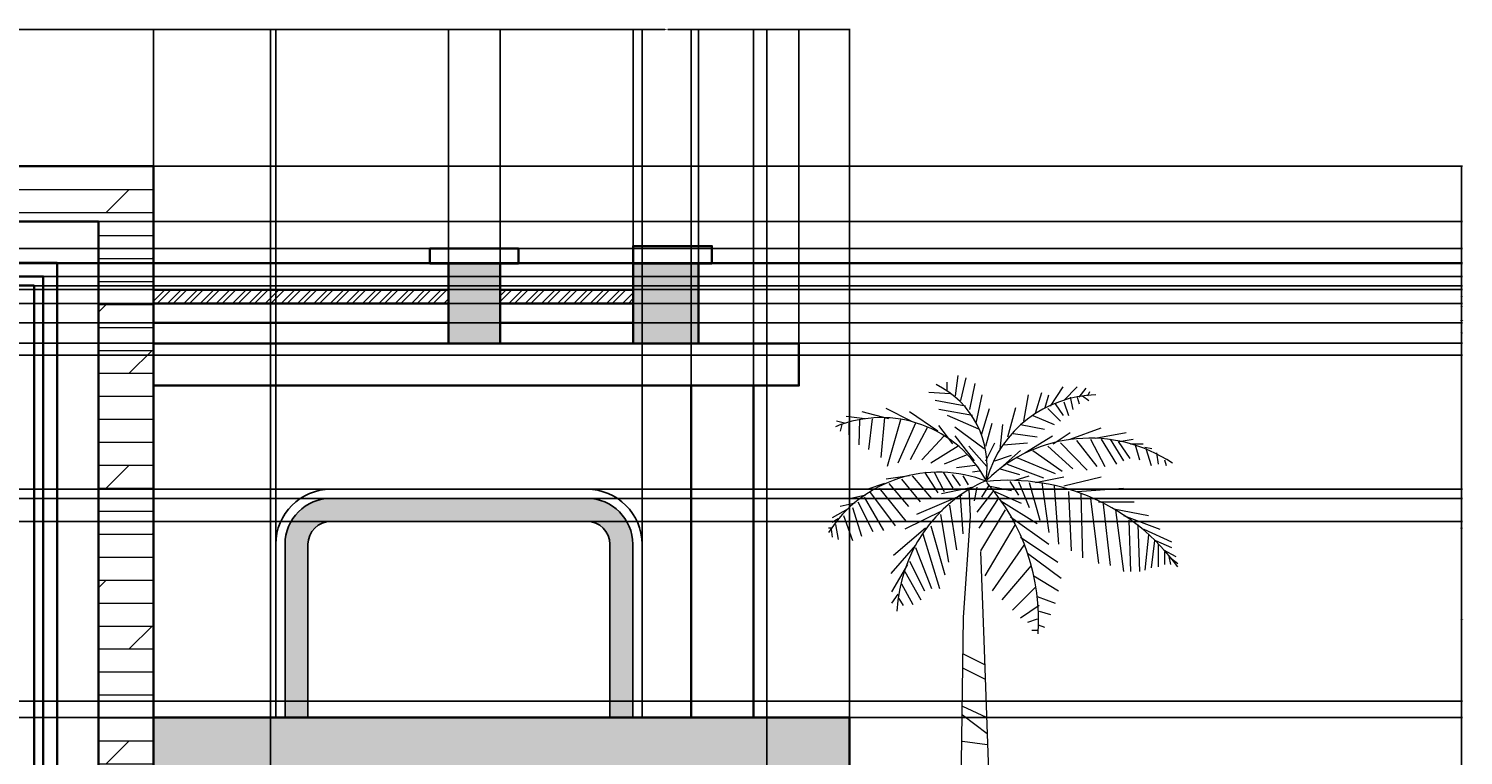
# Model space of a CAD drawing. Units: inches. Extents: x -13 to 630, y -103 to 275.
# Tile 9 of 9: x 318 to 630, y 117 to 275. Entities that reach past the tile are written whole.
import ezdxf

# ---------------------------------------------------------------- set-up
doc = ezdxf.new("R2010")
doc.units = ezdxf.units.IN
doc.header["$MEASUREMENT"] = 0
for name, color, linetype, lineweight in [('A-ANNO-DIMS', 2, 'Continuous', 18), ('A-ELEV', 7, 'Continuous', 35), ('A-ELEV-PATT', 8, 'Continuous', 13), ('A-GLAZ', 4, 'Continuous', 25), ('L-PLNT', 3, 'Continuous', 13)]:
    doc.layers.add(name, color=color, linetype=linetype, lineweight=lineweight)
doc.styles.get("Standard").update_dxf_attribs({"font": 'arial.ttf'})
doc.dimstyles.get("Standard").update_dxf_attribs({"dimtxt": 0.18, "dimasz": 0.18, "dimexe": 0.18, "dimexo": 0.0625, "dimgap": 0.09, "dimtad": 0, "dimtih": 1, "dimtoh": 1, "dimdec": 4, "dimzin": 0, "dimdsep": 46, "dimtxsty": 'Standard', "dimcen": 0.09, "dimadec": 0, "dimazin": 0, "dimtfac": 1, "dimtdec": 4, "dimtofl": 0, "dimtmove": 0, "dimatfit": 3, "dimfxl": 1, "dimtolj": 1, "dimtzin": 0, "dimarcsym": 0})

# ---------------------------------------------------------------- blocks, each defined once
blk = doc.blocks.new('*U2')
for p, q in [((-5.567, 196.707), (-4.987, 201.167)), ((-4.407, 195.716), (-3.247, 200.672)), ((-6.727, 197.202), (-11.366, 197.45)), ((-7.5, 199.68), (-7.5, 197.946)), ((-2.474, 193.733), (-1.315, 199.433)), ((-1.121, 190.759), (0.232, 196.955)), ((9.317, 191.255), (10.283, 196.955)), ((11.829, 192.99), (13.182, 197.45)), ((13.956, 194.229), (14.729, 196.955)), ((15.116, 194.477), (17.822, 198.689)), ((18.015, 195.716), (20.914, 198.689)), ((21.301, 196.459), (22.847, 198.441)), ((22.074, 196.707), (23.427, 195.716)), ((23.234, 196.707), (23.62, 197.698)), ((-15.232, 191.255), (-20.644, 193.981)), ((-3.441, 194.477), (-10.013, 195.716)), ((-1.894, 192.494), (-9.24, 193.733)), ((0.038, 188.281), (1.778, 193.981)), ((5.837, 187.786), (7.577, 194.229)), ((14.536, 193.981), (17.242, 191.255)), ((16.082, 194.972), (17.822, 192.494)), ((18.015, 195.468), (18.981, 192.494)), ((19.368, 196.459), (19.948, 193.733)), ((20.914, 196.459), (21.301, 194.972)), ((-29.729, 190.759), (-31.469, 191.255)), ((-30.309, 190.512), (-30.695, 189.025)), ((-25.283, 191.751), (-29.342, 192.246)), ((-28.763, 190.759), (-28.763, 188.281)), ((-26.443, 191.503), (-26.636, 186.051)), ((-20.064, 191.751), (-25.863, 193.238)), ((-23.737, 191.751), (-24.51, 185.06)), ((-21.031, 191.998), (-21.804, 183.325)), ((-17.551, 191.503), (-20.451, 181.343)), ((-14.265, 190.759), (-18.131, 182.086)), ((-9.433, 189.025), (-15.618, 193.238)), ((-0.541, 189.52), (-7.307, 192.494)), ((1.005, 185.803), (2.358, 190.759)), ((4.098, 185.06), (4.678, 190.512)), ((8.544, 190.512), (13.763, 189.52)), ((11.25, 192.494), (15.889, 190.512)), ((-11.753, 189.768), (-15.425, 182.83)), ((-8.08, 188.034), (-12.912, 182.83)), ((-6.147, 186.299), (-9.24, 190.264)), ((-5.76, 190.016), (0.618, 185.308)), ((-5.76, 188.034), (-1.508, 182.582)), ((6.997, 188.529), (12.216, 187.786)), ((9.51, 184.317), (15.502, 188.034)), ((15.695, 186.299), (19.368, 188.777)), ((19.368, 187.29), (26.133, 189.768)), ((23.814, 187.29), (26.907, 181.343)), ((24.78, 187.538), (31.546, 188.777)), ((26.133, 187.29), (29.419, 181.838)), ((28.066, 187.29), (30.966, 182.582)), ((29.999, 186.795), (33.092, 187.29)), ((-4.987, 185.803), (-10.979, 182.086)), ((-2.668, 185.803), (1.198, 181.343)), ((1.005, 182.582), (2.938, 186.547)), ((4.871, 186.051), (10.09, 186.547)), ((4.871, 181.591), (8.544, 184.812)), ((11.25, 184.812), (17.628, 180.352)), ((14.536, 185.803), (19.948, 180.847)), ((17.242, 186.547), (23.041, 180.599)), ((20.721, 187.042), (25.167, 181.343)), ((29.806, 186.795), (32.319, 183.078)), ((32.512, 186.299), (35.218, 186.299)), ((33.479, 186.051), (34.445, 182.83)), ((35.605, 185.556), (37.151, 185.308)), ((35.798, 185.308), (36.958, 181.591)), ((38.118, 184.317), (38.504, 181.838)), ((-3.247, 183.821), (-8.08, 181.838)), ((-1.315, 181.591), (-5.374, 181.095)), ((2.938, 182.582), (6.61, 183.821)), ((5.644, 181.838), (13.569, 178.865)), ((7.77, 183.325), (16.082, 179.856)), ((39.857, 182.83), (40.244, 181.591)), ((-15.618, 179.36), (-20.644, 178.617)), ((-17.358, 178.617), (-13.299, 173.661)), ((-15.038, 179.36), (-10.786, 174.404)), ((-12.332, 180.104), (-9.433, 175.643)), ((-10.206, 180.104), (-8.08, 175.891)), ((-8.273, 180.104), (-6.147, 176.635)), ((-6.34, 179.608), (-4.6, 177.13)), ((-4.021, 179.36), (-2.861, 177.378)), ((-0.348, 180.352), (-1.894, 180.104)), ((4.098, 180.847), (8.35, 179.608)), ((6.224, 178.121), (8.157, 175.148)), ((7.384, 178.369), (10.476, 179.36)), ((8.157, 178.121), (10.476, 172.422)), ((11.829, 177.874), (18.015, 179.113)), ((18.015, 177.13), (26.133, 179.113)), ((-25.09, 175.148), (-28.376, 174.404)), ((-21.031, 177.626), (-24.897, 176.387)), ((-24.317, 175.891), (-18.711, 168.457)), ((-22.191, 176.635), (-16.391, 169.448)), ((-20.064, 177.626), (-15.812, 172.67)), ((-4.214, 175.148), (-14.072, 170.935)), ((-1.701, 176.882), (-8.66, 175.396)), ((-4.6, 174.9), (-4.021, 166.722)), ((-2.668, 176.387), (-2.376, 170.594)), ((-0.928, 176.882), (-1.508, 173.909)), ((2.551, 175.891), (-0.928, 171.431)), ((1.585, 177.13), (0.038, 174.652)), ((1.585, 177.13), (6.61, 176.139)), ((2.938, 175.891), (8.737, 173.413)), ((10.476, 177.874), (12.796, 169.696)), ((13.182, 177.874), (14.729, 166.97)), ((15.889, 177.13), (16.855, 164.492)), ((18.981, 175.891), (19.561, 163.005)), ((20.914, 175.891), (30.966, 176.635)), ((21.688, 175.396), (22.074, 161.518)), ((-28.956, 172.174), (-32.435, 170.192)), ((-27.409, 173.413), (-30.695, 172.67)), ((-27.989, 172.422), (-26.056, 166.227)), ((-26.829, 173.661), (-23.544, 167.218)), ((-25.476, 174.652), (-21.224, 167.466)), ((-8.466, 171.678), (-16.585, 167.713)), ((-6.92, 172.917), (-5.374, 163.253)), ((3.711, 174.404), (-0.541, 167.961)), ((5.257, 171.926), (-0.155, 163.005)), ((4.291, 173.909), (12.216, 168.953)), ((23.814, 174.404), (25.554, 160.279)), ((25.554, 173.661), (33.285, 173.661)), ((26.52, 173.165), (28.066, 159.784)), ((28.839, 172.174), (36.378, 170.687)), ((29.226, 171.926), (30.966, 158.545)), ((-31.082, 169.944), (-32.435, 169.2)), ((-31.662, 168.705), (-31.082, 165.483)), ((-29.922, 170.687), (-27.989, 165.235)), ((-8.853, 170.935), (-7.113, 160.527)), ((7.384, 168.705), (0.812, 157.553)), ((6.417, 170.439), (14.729, 164.492)), ((30.966, 170.687), (38.891, 167.713)), ((32.126, 169.696), (32.512, 158.545)), ((34.058, 168.705), (34.445, 158.545)), ((-32.628, 167.961), (-33.208, 167.961)), ((-32.628, 167.713), (-32.435, 165.979)), ((-12.139, 167.961), (-19.098, 162.014)), ((-12.719, 166.722), (-9.046, 154.828)), ((-10.979, 168.457), (-7.887, 157.801)), ((8.544, 165.979), (16.662, 160.527)), ((35.412, 167.713), (41.404, 164.988)), ((36.378, 166.474), (35.605, 158.792)), ((-14.265, 164.244), (-19.678, 158.049)), ((-14.265, 163.749), (-10.786, 154.828)), ((9.317, 164.244), (2.358, 154.332)), ((10.09, 162.51), (17.435, 157.058)), ((37.731, 165.235), (36.958, 159.288)), ((37.924, 165.235), (41.404, 163.749)), ((38.504, 164.492), (38.504, 159.536)), ((39.664, 163.253), (42.37, 161.766)), ((39.857, 162.757), (39.857, 160.031)), ((-16.005, 160.031), (-19.484, 154.084)), ((-15.618, 160.775), (-12.332, 154.332)), ((10.863, 159.784), (4.484, 152.35)), ((40.824, 161.766), (41.21, 160.031)), ((41.21, 161.518), (42.757, 160.279)), ((-16.585, 158.545), (-13.106, 152.35)), ((11.443, 157.553), (16.855, 154.332)), ((-18.131, 153.589), (-19.484, 151.606)), ((-17.358, 155.819), (-14.845, 151.358)), ((11.829, 155.075), (6.804, 150.119)), ((12.216, 153.093), (16.082, 151.606)), ((-17.938, 152.597), (-16.972, 151.111)), ((12.603, 151.111), (8.544, 148.385)), ((12.603, 149.872), (15.116, 149.128)), ((12.216, 148.137), (10.09, 147.393)), ((12.409, 146.898), (13.763, 146.402)), ((12.409, 145.659), (11.056, 145.659)), ((-4.081, 140.645), (0.753, 138.261)), ((-4.081, 137.547), (0.753, 135.163)), ((-4.081, 129.205), (1.124, 126.821)), ((-4.081, 127.298), (1.31, 123.246)), ((-4.081, 121.578), (1.31, 120.863))]:
    blk.add_line(p, q)
for points in [[(-2.363, 170.553), (-3.88, 148.505), (-4.988, 69.634), (-3.325, 24.869), (0, 0)], [(-0.116, 162.848), (0.554, 143.532), (2.217, 96.635), (3.88, 44.054), (7.76, 12.079), (11.64, 0)]]:
    blk.add_lwpolyline(points)
for centre, radius, start, end in [((-18.427, 181.448), 19.715, 350.285, 64.11229), ((25.595, 171.567), 25.395, 91.40319, 163.882), ((-21.738, 166.094), 25.899, 27.67115, 112.5305), ((23.687, 155.341), 32.188, 56.19272, 134.3213), ((-9.259, 151.732), 28.386, 68.38311, 147.5322), ((14.394, 148.393), 32.752, 113.7592, 177.4133), ((5.828, 132.718), 45.639, 35.98777, 95.82273), ((-32.8, 147.923), 45.309, 356.1943, 41.37848)]:
    blk.add_arc(centre, radius, start, end)
blk = doc.blocks.new('*D9')
at = {"layer": 'A-ANNO-DIMS', "color": 0, "lineweight": -2, "transparency": 16777216}
for p, q in [((345.31, 5.14), (345.31, 275.01)), ((345.49, 274.83), (357.54, 274.83)), ((370.53, 274.83), (358.47, 274.83)), ((370.71, 5.14), (370.71, 275.01))]:
    blk.add_line(p, q, dxfattribs=at)
at = {"layer": 'A-ANNO-DIMS', "color": 0, "transparency": 16777216}
for points in [[(345.49, 274.86), (345.49, 274.8), (345.31, 274.83)], [(370.53, 274.86), (370.53, 274.8), (370.71, 274.83)]]:
    blk.add_solid(points, dxfattribs=at)
at = {"layer": 'Defpoints', "color": 0, "transparency": 16777216}
for p in [(370.71, 274.83), (345.31, 5.08), (370.71, 5.08)]:
    blk.add_point(p, dxfattribs=at)
at = {"layer": 'A-ANNO-DIMS', "color": 0, "transparency": 16777216, "insert": (358.01, 274.83), "char_height": 0.18, "attachment_point": 5}
blk.add_mtext('\\A1;25.406', dxfattribs=at)
blk = doc.blocks.new('*D10')
at = {"layer": 'A-ANNO-DIMS', "color": 0, "lineweight": -2, "transparency": 16777216}
for p, q in [((478.71, 107.14), (478.71, 275.01)), ((478.89, 274.83), (487.5, 274.83)), ((496.53, 274.83), (487.92, 274.83)), ((496.71, 125.14), (496.71, 275.01))]:
    blk.add_line(p, q, dxfattribs=at)
at = {"layer": 'A-ANNO-DIMS', "color": 0, "transparency": 16777216}
for points in [[(478.89, 274.86), (478.89, 274.8), (478.71, 274.83)], [(496.53, 274.86), (496.53, 274.8), (496.71, 274.83)]]:
    blk.add_solid(points, dxfattribs=at)
at = {"layer": 'Defpoints', "color": 0, "transparency": 16777216}
for p in [(496.71, 274.83), (496.71, 125.08), (478.71, 107.08)]:
    blk.add_point(p, dxfattribs=at)
at = {"layer": 'A-ANNO-DIMS', "color": 0, "transparency": 16777216, "insert": (487.71, 274.83), "char_height": 0.18, "attachment_point": 5}
blk.add_mtext('\\A1;18', dxfattribs=at)
blk = doc.blocks.new('*D13')
at = {"layer": 'A-ANNO-DIMS', "color": 0, "lineweight": -2, "transparency": 16777216}
for p, q in [((345.37, 245.08), (630.03, 245.08)), ((629.85, 244.9), (629.85, 125.26)), ((629.85, 5.26), (629.85, 124.9)), ((496.77, 5.08), (630.03, 5.08))]:
    blk.add_line(p, q, dxfattribs=at)
at = {"layer": 'A-ANNO-DIMS', "color": 0, "transparency": 16777216}
for points in [[(629.82, 244.9), (629.88, 244.9), (629.85, 245.08)], [(629.82, 5.26), (629.88, 5.26), (629.85, 5.08)]]:
    blk.add_solid(points, dxfattribs=at)
at = {"layer": 'Defpoints', "color": 0, "transparency": 16777216}
for p in [(345.31, 245.08), (629.85, 245.08), (496.71, 5.08)]:
    blk.add_point(p, dxfattribs=at)
at = {"layer": 'A-ANNO-DIMS', "color": 0, "transparency": 16777216, "insert": (629.85, 125.08), "char_height": 0.18, "attachment_point": 5}
blk.add_mtext('\\A1;240', dxfattribs=at)
blk = doc.blocks.new('*D14')
at = {"layer": 'A-ANNO-DIMS', "color": 0, "lineweight": -2, "transparency": 16777216}
for p, q in [((345.31, 206.59), (345.31, 275.01)), ((345.49, 274.83), (376.97, 274.83)), ((409.25, 274.83), (377.76, 274.83)), ((409.43, 206.59), (409.43, 275.01))]:
    blk.add_line(p, q, dxfattribs=at)
at = {"layer": 'A-ANNO-DIMS', "color": 0, "transparency": 16777216}
for points in [[(345.49, 274.86), (345.49, 274.8), (345.31, 274.83)], [(409.25, 274.86), (409.25, 274.8), (409.43, 274.83)]]:
    blk.add_solid(points, dxfattribs=at)
at = {"layer": 'Defpoints', "color": 0, "transparency": 16777216}
for p in [(409.43, 274.83), (345.31, 206.53), (409.43, 206.53)]:
    blk.add_point(p, dxfattribs=at)
at = {"layer": 'A-ANNO-DIMS', "color": 0, "transparency": 16777216, "insert": (377.37, 274.83), "char_height": 0.18, "attachment_point": 5}
blk.add_mtext('\\A1;64.12', dxfattribs=at)
blk = doc.blocks.new('*D15')
at = {"layer": 'A-ANNO-DIMS', "color": 0, "lineweight": -2, "transparency": 16777216}
for p, q in [((409.43, 206.59), (409.43, 275.01)), ((409.61, 274.83), (414.6, 274.83)), ((420.5, 274.83), (415.51, 274.83)), ((420.68, 206.59), (420.68, 275.01))]:
    blk.add_line(p, q, dxfattribs=at)
at = {"layer": 'A-ANNO-DIMS', "color": 0, "transparency": 16777216}
for points in [[(409.61, 274.86), (409.61, 274.8), (409.43, 274.83)], [(420.5, 274.86), (420.5, 274.8), (420.68, 274.83)]]:
    blk.add_solid(points, dxfattribs=at)
at = {"layer": 'Defpoints', "color": 0, "transparency": 16777216}
for p in [(420.68, 274.83), (409.43, 206.53), (420.68, 206.53)]:
    blk.add_point(p, dxfattribs=at)
at = {"layer": 'A-ANNO-DIMS', "color": 0, "transparency": 16777216, "insert": (415.06, 274.83), "char_height": 0.18, "attachment_point": 5}
blk.add_mtext('\\A1;11.255', dxfattribs=at)
blk = doc.blocks.new('*D16')
at = {"layer": 'A-ANNO-DIMS', "color": 0, "lineweight": -2, "transparency": 16777216}
for p, q in [((420.68, 206.59), (420.68, 275.01)), ((420.86, 274.83), (434.76, 274.83)), ((449.45, 274.83), (435.55, 274.83)), ((449.63, 206.59), (449.63, 275.01))]:
    blk.add_line(p, q, dxfattribs=at)
at = {"layer": 'A-ANNO-DIMS', "color": 0, "transparency": 16777216}
for points in [[(420.86, 274.86), (420.86, 274.8), (420.68, 274.83)], [(449.45, 274.86), (449.45, 274.8), (449.63, 274.83)]]:
    blk.add_solid(points, dxfattribs=at)
at = {"layer": 'Defpoints', "color": 0, "transparency": 16777216}
for p in [(449.63, 274.83), (420.68, 206.53), (449.63, 206.53)]:
    blk.add_point(p, dxfattribs=at)
at = {"layer": 'A-ANNO-DIMS', "color": 0, "transparency": 16777216, "insert": (435.15, 274.83), "char_height": 0.18, "attachment_point": 5}
blk.add_mtext('\\A1;28.94', dxfattribs=at)
blk = doc.blocks.new('*D17')
at = {"layer": 'A-ANNO-DIMS', "color": 0, "lineweight": -2, "transparency": 16777216}
for p, q in [((449.63, 206.59), (449.63, 275.01)), ((449.81, 274.83), (456.27, 274.83)), ((463.65, 274.83), (457.18, 274.83)), ((463.83, 206.59), (463.83, 275.01))]:
    blk.add_line(p, q, dxfattribs=at)
at = {"layer": 'A-ANNO-DIMS', "color": 0, "transparency": 16777216}
for points in [[(449.81, 274.86), (449.81, 274.8), (449.63, 274.83)], [(463.65, 274.86), (463.65, 274.8), (463.83, 274.83)]]:
    blk.add_solid(points, dxfattribs=at)
at = {"layer": 'Defpoints', "color": 0, "transparency": 16777216}
for p in [(463.83, 274.83), (449.63, 206.53), (463.83, 206.53)]:
    blk.add_point(p, dxfattribs=at)
at = {"layer": 'A-ANNO-DIMS', "color": 0, "transparency": 16777216, "insert": (456.73, 274.83), "char_height": 0.18, "attachment_point": 5}
blk.add_mtext('\\A1;14.203', dxfattribs=at)
blk = doc.blocks.new('*D18')
at = {"layer": 'A-ANNO-DIMS', "color": 0, "lineweight": -2, "transparency": 16777216}
for p, q in [((463.83, 206.59), (463.83, 275.01)), ((464.01, 274.83), (474.28, 274.83)), ((485.49, 274.83), (475.22, 274.83)), ((485.67, 206.59), (485.67, 275.01))]:
    blk.add_line(p, q, dxfattribs=at)
at = {"layer": 'A-ANNO-DIMS', "color": 0, "transparency": 16777216}
for points in [[(464.01, 274.86), (464.01, 274.8), (463.83, 274.83)], [(485.49, 274.86), (485.49, 274.8), (485.67, 274.83)]]:
    blk.add_solid(points, dxfattribs=at)
at = {"layer": 'Defpoints', "color": 0, "transparency": 16777216}
for p in [(485.67, 274.83), (463.83, 206.53), (485.67, 206.53)]:
    blk.add_point(p, dxfattribs=at)
at = {"layer": 'A-ANNO-DIMS', "color": 0, "transparency": 16777216, "insert": (474.75, 274.83), "char_height": 0.18, "attachment_point": 5}
blk.add_mtext('\\A1;21.845', dxfattribs=at)
blk = doc.blocks.new('*D19')
at = {"layer": 'A-ANNO-DIMS', "color": 0, "lineweight": -2, "transparency": 16777216}
for p, q in [((485.67, 206.59), (485.67, 275.01)), ((485.85, 274.83), (490.74, 274.83)), ((496.53, 274.83), (491.65, 274.83)), ((496.71, 125.14), (496.71, 275.01))]:
    blk.add_line(p, q, dxfattribs=at)
at = {"layer": 'A-ANNO-DIMS', "color": 0, "transparency": 16777216}
for points in [[(485.85, 274.86), (485.85, 274.8), (485.67, 274.83)], [(496.53, 274.86), (496.53, 274.8), (496.71, 274.83)]]:
    blk.add_solid(points, dxfattribs=at)
at = {"layer": 'Defpoints', "color": 0, "transparency": 16777216}
for p in [(496.71, 274.83), (485.67, 206.53), (496.71, 125.08)]:
    blk.add_point(p, dxfattribs=at)
at = {"layer": 'A-ANNO-DIMS', "color": 0, "transparency": 16777216, "insert": (491.19, 274.83), "char_height": 0.18, "attachment_point": 5}
blk.add_mtext('\\A1;11.038', dxfattribs=at)
blk = doc.blocks.new('*D20')
at = {"layer": 'A-ANNO-DIMS', "color": 0, "lineweight": -2, "transparency": 16777216}
for p, q in [((345.31, 125.14), (345.31, 275.01)), ((345.49, 274.83), (358.13, 274.83)), ((371.7, 274.83), (359.06, 274.83)), ((371.88, 125.14), (371.88, 275.01))]:
    blk.add_line(p, q, dxfattribs=at)
at = {"layer": 'A-ANNO-DIMS', "color": 0, "transparency": 16777216}
for points in [[(345.49, 274.86), (345.49, 274.8), (345.31, 274.83)], [(371.7, 274.86), (371.7, 274.8), (371.88, 274.83)]]:
    blk.add_solid(points, dxfattribs=at)
at = {"layer": 'Defpoints', "color": 0, "transparency": 16777216}
for p in [(371.88, 274.83), (345.31, 125.08), (371.88, 125.08)]:
    blk.add_point(p, dxfattribs=at)
at = {"layer": 'A-ANNO-DIMS', "color": 0, "transparency": 16777216, "insert": (358.59, 274.83), "char_height": 0.18, "attachment_point": 5}
blk.add_mtext('\\A1;26.576', dxfattribs=at)
blk = doc.blocks.new('*D21')
at = {"layer": 'A-ANNO-DIMS', "color": 0, "lineweight": -2, "transparency": 16777216}
for p, q in [((371.88, 125.14), (371.88, 275.01)), ((372.06, 274.83), (411.32, 274.83)), ((451.37, 274.83), (412.11, 274.83)), ((451.55, 125.14), (451.55, 275.01))]:
    blk.add_line(p, q, dxfattribs=at)
at = {"layer": 'A-ANNO-DIMS', "color": 0, "transparency": 16777216}
for points in [[(372.06, 274.86), (372.06, 274.8), (371.88, 274.83)], [(451.37, 274.86), (451.37, 274.8), (451.55, 274.83)]]:
    blk.add_solid(points, dxfattribs=at)
at = {"layer": 'Defpoints', "color": 0, "transparency": 16777216}
for p in [(451.55, 274.83), (371.88, 125.08), (451.55, 125.08)]:
    blk.add_point(p, dxfattribs=at)
at = {"layer": 'A-ANNO-DIMS', "color": 0, "transparency": 16777216, "insert": (411.72, 274.83), "char_height": 0.18, "attachment_point": 5}
blk.add_mtext('\\A1;79.67', dxfattribs=at)
blk = doc.blocks.new('*D22')
at = {"layer": 'A-ANNO-DIMS', "color": 0, "lineweight": -2, "transparency": 16777216}
for p, q in [((451.55, 125.14), (451.55, 275.01)), ((451.73, 274.83), (456.54, 274.83)), ((462.08, 274.83), (457.27, 274.83)), ((462.26, 125.14), (462.26, 275.01))]:
    blk.add_line(p, q, dxfattribs=at)
at = {"layer": 'A-ANNO-DIMS', "color": 0, "transparency": 16777216}
for points in [[(451.73, 274.86), (451.73, 274.8), (451.55, 274.83)], [(462.08, 274.86), (462.08, 274.8), (462.26, 274.83)]]:
    blk.add_solid(points, dxfattribs=at)
at = {"layer": 'Defpoints', "color": 0, "transparency": 16777216}
for p in [(462.26, 274.83), (451.55, 125.08), (462.26, 125.08)]:
    blk.add_point(p, dxfattribs=at)
at = {"layer": 'A-ANNO-DIMS', "color": 0, "transparency": 16777216, "insert": (456.91, 274.83), "char_height": 0.18, "attachment_point": 5}
blk.add_mtext('\\A1;10.71', dxfattribs=at)
blk = doc.blocks.new('*D23')
at = {"layer": 'A-ANNO-DIMS', "color": 0, "lineweight": -2, "transparency": 16777216}
for p, q in [((462.26, 125.14), (462.26, 275.01)), ((462.44, 274.83), (468.59, 274.83)), ((475.65, 274.83), (469.5, 274.83)), ((475.83, 125.14), (475.83, 275.01))]:
    blk.add_line(p, q, dxfattribs=at)
at = {"layer": 'A-ANNO-DIMS', "color": 0, "transparency": 16777216}
for points in [[(462.44, 274.86), (462.44, 274.8), (462.26, 274.83)], [(475.65, 274.86), (475.65, 274.8), (475.83, 274.83)]]:
    blk.add_solid(points, dxfattribs=at)
at = {"layer": 'Defpoints', "color": 0, "transparency": 16777216}
for p in [(475.83, 274.83), (462.26, 125.08), (475.83, 125.08)]:
    blk.add_point(p, dxfattribs=at)
at = {"layer": 'A-ANNO-DIMS', "color": 0, "transparency": 16777216, "insert": (469.05, 274.83), "char_height": 0.18, "attachment_point": 5}
blk.add_mtext('\\A1;13.574', dxfattribs=at)
blk = doc.blocks.new('*D27')
at = {"layer": 'A-ANNO-DIMS', "color": 0, "lineweight": -2, "transparency": 16777216}
for p, q in [((164.84, 245.14), (164.84, 275.01)), ((165.02, 274.83), (254.62, 274.83)), ((345.13, 274.83), (255.53, 274.83)), ((345.31, 245.14), (345.31, 275.01))]:
    blk.add_line(p, q, dxfattribs=at)
at = {"layer": 'A-ANNO-DIMS', "color": 0, "transparency": 16777216}
for points in [[(165.02, 274.86), (165.02, 274.8), (164.84, 274.83)], [(345.13, 274.86), (345.13, 274.8), (345.31, 274.83)]]:
    blk.add_solid(points, dxfattribs=at)
at = {"layer": 'Defpoints', "color": 0, "transparency": 16777216}
for p in [(345.31, 274.83), (164.84, 245.08), (345.31, 245.08)]:
    blk.add_point(p, dxfattribs=at)
at = {"layer": 'A-ANNO-DIMS', "color": 0, "transparency": 16777216, "insert": (255.08, 274.83), "char_height": 0.18, "attachment_point": 5}
blk.add_mtext('\\A1;180.46', dxfattribs=at)
blk = doc.blocks.new('*D28')
at = {"layer": 'A-ANNO-DIMS', "color": 0, "lineweight": -2, "transparency": 16777216}
for p, q in [((302.59, 128.66), (630.03, 128.66)), ((629.85, 128.48), (629.85, 67.05)), ((629.85, 5.26), (629.85, 66.69)), ((302.59, 5.08), (630.03, 5.08))]:
    blk.add_line(p, q, dxfattribs=at)
at = {"layer": 'A-ANNO-DIMS', "color": 0, "transparency": 16777216}
for points in [[(629.82, 128.48), (629.88, 128.48), (629.85, 128.66)], [(629.82, 5.26), (629.88, 5.26), (629.85, 5.08)]]:
    blk.add_solid(points, dxfattribs=at)
at = {"layer": 'Defpoints', "color": 0, "transparency": 16777216}
for p in [(302.53, 128.66), (629.85, 128.66), (302.53, 5.08)]:
    blk.add_point(p, dxfattribs=at)
at = {"layer": 'A-ANNO-DIMS', "color": 0, "transparency": 16777216, "insert": (629.85, 66.87), "char_height": 0.18, "attachment_point": 5}
blk.add_mtext('\\A1;123.57', dxfattribs=at)
blk = doc.blocks.new('*D29')
at = {"layer": 'A-ANNO-DIMS', "color": 0, "lineweight": -2, "transparency": 16777216}
for p, q in [((302.59, 203.94), (630.03, 203.94)), ((629.85, 203.76), (629.85, 166.48)), ((629.85, 128.84), (629.85, 166.11)), ((302.59, 128.66), (630.03, 128.66))]:
    blk.add_line(p, q, dxfattribs=at)
at = {"layer": 'A-ANNO-DIMS', "color": 0, "transparency": 16777216}
for points in [[(629.82, 203.76), (629.88, 203.76), (629.85, 203.94)], [(629.82, 128.84), (629.88, 128.84), (629.85, 128.66)]]:
    blk.add_solid(points, dxfattribs=at)
at = {"layer": 'Defpoints', "color": 0, "transparency": 16777216}
for p in [(302.53, 203.94), (629.85, 203.94), (302.53, 128.66)]:
    blk.add_point(p, dxfattribs=at)
at = {"layer": 'A-ANNO-DIMS', "color": 0, "transparency": 16777216, "insert": (629.85, 166.3), "char_height": 0.18, "attachment_point": 5}
blk.add_mtext('\\A1;75.28', dxfattribs=at)
blk = doc.blocks.new('*D35')
at = {"layer": 'A-ANNO-DIMS', "color": 0, "lineweight": -2, "transparency": 16777216}
for p, q in [((319.37, 219.08), (630.03, 219.08)), ((629.85, 218.9), (629.85, 211.69)), ((629.85, 204.12), (629.85, 211.33)), ((302.59, 203.94), (630.03, 203.94))]:
    blk.add_line(p, q, dxfattribs=at)
at = {"layer": 'A-ANNO-DIMS', "color": 0, "transparency": 16777216}
for points in [[(629.82, 218.9), (629.88, 218.9), (629.85, 219.08)], [(629.82, 204.12), (629.88, 204.12), (629.85, 203.94)]]:
    blk.add_solid(points, dxfattribs=at)
at = {"layer": 'Defpoints', "color": 0, "transparency": 16777216}
for p in [(319.31, 219.08), (629.85, 219.08), (302.53, 203.94)]:
    blk.add_point(p, dxfattribs=at)
at = {"layer": 'A-ANNO-DIMS', "color": 0, "transparency": 16777216, "insert": (629.85, 211.51), "char_height": 0.18, "attachment_point": 5}
blk.add_mtext('\\A1;15.145', dxfattribs=at)
blk = doc.blocks.new('*D36')
at = {"layer": 'A-ANNO-DIMS', "color": 0, "lineweight": -2, "transparency": 16777216}
for p, q in [((319.37, 219.08), (630.03, 219.08)), ((321.37, 221.08), (630.03, 221.08)), ((629.85, 220.9), (629.85, 220.26)), ((629.85, 219.26), (629.85, 219.9))]:
    blk.add_line(p, q, dxfattribs=at)
at = {"layer": 'A-ANNO-DIMS', "color": 0, "transparency": 16777216}
for points in [[(629.82, 220.9), (629.88, 220.9), (629.85, 221.08)], [(629.82, 219.26), (629.88, 219.26), (629.85, 219.08)]]:
    blk.add_solid(points, dxfattribs=at)
at = {"layer": 'Defpoints', "color": 0, "transparency": 16777216}
for p in [(319.31, 219.08), (321.31, 221.08), (629.85, 221.08)]:
    blk.add_point(p, dxfattribs=at)
at = {"layer": 'A-ANNO-DIMS', "color": 0, "transparency": 16777216, "insert": (629.85, 220.08), "char_height": 0.18, "attachment_point": 5}
blk.add_mtext('\\A1;2', dxfattribs=at)
blk = doc.blocks.new('*D37')
at = {"layer": 'A-ANNO-DIMS', "color": 0, "lineweight": -2, "transparency": 16777216}
for p, q in [((324.37, 224.08), (630.03, 224.08)), ((629.85, 223.9), (629.85, 222.76)), ((629.85, 221.26), (629.85, 222.4)), ((321.37, 221.08), (630.03, 221.08))]:
    blk.add_line(p, q, dxfattribs=at)
at = {"layer": 'A-ANNO-DIMS', "color": 0, "transparency": 16777216}
for points in [[(629.82, 223.9), (629.88, 223.9), (629.85, 224.08)], [(629.82, 221.26), (629.88, 221.26), (629.85, 221.08)]]:
    blk.add_solid(points, dxfattribs=at)
at = {"layer": 'Defpoints', "color": 0, "transparency": 16777216}
for p in [(324.31, 224.08), (629.85, 224.08), (321.31, 221.08)]:
    blk.add_point(p, dxfattribs=at)
at = {"layer": 'A-ANNO-DIMS', "color": 0, "transparency": 16777216, "insert": (629.85, 222.58), "char_height": 0.18, "attachment_point": 5}
blk.add_mtext('\\A1;3', dxfattribs=at)
blk = doc.blocks.new('*D38')
at = {"layer": 'A-ANNO-DIMS', "color": 0, "lineweight": -2, "transparency": 16777216}
for p, q in [((333.37, 233.08), (630.03, 233.08)), ((629.85, 232.9), (629.85, 228.76)), ((629.85, 224.26), (629.85, 228.4)), ((324.37, 224.08), (630.03, 224.08))]:
    blk.add_line(p, q, dxfattribs=at)
at = {"layer": 'A-ANNO-DIMS', "color": 0, "transparency": 16777216}
for points in [[(629.82, 232.9), (629.88, 232.9), (629.85, 233.08)], [(629.82, 224.26), (629.88, 224.26), (629.85, 224.08)]]:
    blk.add_solid(points, dxfattribs=at)
at = {"layer": 'Defpoints', "color": 0, "transparency": 16777216}
for p in [(333.31, 233.08), (629.85, 233.08), (324.31, 224.08)]:
    blk.add_point(p, dxfattribs=at)
at = {"layer": 'A-ANNO-DIMS', "color": 0, "transparency": 16777216, "insert": (629.85, 228.58), "char_height": 0.18, "attachment_point": 5}
blk.add_mtext('\\A1;9', dxfattribs=at)
blk = doc.blocks.new('*D39')
at = {"layer": 'A-ANNO-DIMS', "color": 0, "lineweight": -2, "transparency": 16777216}
for p, q in [((345.37, 245.08), (630.03, 245.08)), ((629.85, 244.9), (629.85, 239.26)), ((629.85, 233.26), (629.85, 238.9)), ((333.37, 233.08), (630.03, 233.08))]:
    blk.add_line(p, q, dxfattribs=at)
at = {"layer": 'A-ANNO-DIMS', "color": 0, "transparency": 16777216}
for points in [[(629.82, 244.9), (629.88, 244.9), (629.85, 245.08)], [(629.82, 233.26), (629.88, 233.26), (629.85, 233.08)]]:
    blk.add_solid(points, dxfattribs=at)
at = {"layer": 'Defpoints', "color": 0, "transparency": 16777216}
for p in [(345.31, 245.08), (629.85, 245.08), (333.31, 233.08)]:
    blk.add_point(p, dxfattribs=at)
at = {"layer": 'A-ANNO-DIMS', "color": 0, "transparency": 16777216, "insert": (629.85, 239.08), "char_height": 0.18, "attachment_point": 5}
blk.add_mtext('\\A1;12', dxfattribs=at)
blk = doc.blocks.new('*D89')
at = {"layer": 'A-ANNO-DIMS', "color": 0, "lineweight": -2, "transparency": 16777216}
for p, q in [((95.18, 210.97), (630.03, 210.97)), ((629.85, 210.79), (629.85, 208.93)), ((95.18, 206.53), (630.03, 206.53)), ((629.85, 206.71), (629.85, 208.57))]:
    blk.add_line(p, q, dxfattribs=at)
at = {"layer": 'A-ANNO-DIMS', "color": 0, "transparency": 16777216}
for points in [[(629.82, 210.79), (629.88, 210.79), (629.85, 210.97)], [(629.82, 206.71), (629.88, 206.71), (629.85, 206.53)]]:
    blk.add_solid(points, dxfattribs=at)
at = {"layer": 'Defpoints', "color": 0, "transparency": 16777216}
for p in [(95.12, 210.97), (629.85, 210.97), (95.12, 206.53)]:
    blk.add_point(p, dxfattribs=at)
at = {"layer": 'A-ANNO-DIMS', "color": 0, "transparency": 16777216, "insert": (629.85, 208.75), "char_height": 0.18, "attachment_point": 5}
blk.add_mtext('\\A1;4.442', dxfattribs=at)
blk = doc.blocks.new('*D90')
at = {"layer": 'A-ANNO-DIMS', "color": 0, "lineweight": -2, "transparency": 16777216}
for p, q in [((95.18, 218.21), (630.03, 218.21)), ((629.85, 218.03), (629.85, 214.77)), ((629.85, 211.15), (629.85, 214.41)), ((95.18, 210.97), (630.03, 210.97))]:
    blk.add_line(p, q, dxfattribs=at)
at = {"layer": 'A-ANNO-DIMS', "color": 0, "transparency": 16777216}
for points in [[(629.82, 218.03), (629.88, 218.03), (629.85, 218.21)], [(629.82, 211.15), (629.88, 211.15), (629.85, 210.97)]]:
    blk.add_solid(points, dxfattribs=at)
at = {"layer": 'Defpoints', "color": 0, "transparency": 16777216}
for p in [(95.12, 218.21), (629.85, 218.21), (95.12, 210.97)]:
    blk.add_point(p, dxfattribs=at)
at = {"layer": 'A-ANNO-DIMS', "color": 0, "transparency": 16777216, "insert": (629.85, 214.59), "char_height": 0.18, "attachment_point": 5}
blk.add_mtext('\\A1;7.236', dxfattribs=at)
blk = doc.blocks.new('*D91')
at = {"layer": 'A-ANNO-DIMS', "color": 0, "lineweight": -2, "transparency": 16777216}
for p, q in [((54.98, 218.21), (630.03, 218.21)), ((629.85, 218.03), (629.85, 216.9)), ((629.85, 215.41), (629.85, 216.54)), ((54.98, 215.23), (630.03, 215.23))]:
    blk.add_line(p, q, dxfattribs=at)
at = {"layer": 'A-ANNO-DIMS', "color": 0, "transparency": 16777216}
for points in [[(629.82, 218.03), (629.88, 218.03), (629.85, 218.21)], [(629.82, 215.41), (629.88, 215.41), (629.85, 215.23)]]:
    blk.add_solid(points, dxfattribs=at)
at = {"layer": 'Defpoints', "color": 0, "transparency": 16777216}
for p in [(54.92, 218.21), (629.85, 218.21), (54.92, 215.23)]:
    blk.add_point(p, dxfattribs=at)
at = {"layer": 'A-ANNO-DIMS', "color": 0, "transparency": 16777216, "insert": (629.85, 216.72), "char_height": 0.18, "attachment_point": 5}
blk.add_mtext('\\A1;2.972', dxfattribs=at)
blk = doc.blocks.new('*D94')
at = {"layer": 'A-ANNO-DIMS', "color": 0, "lineweight": -2, "transparency": 16777216}
for p, q in [((99.2, 227.15), (630.03, 227.15)), ((629.85, 226.97), (629.85, 225.73)), ((629.85, 224.12), (629.85, 225.36)), ((99.2, 223.94), (630.03, 223.94))]:
    blk.add_line(p, q, dxfattribs=at)
at = {"layer": 'A-ANNO-DIMS', "color": 0, "transparency": 16777216}
for points in [[(629.82, 226.97), (629.88, 226.97), (629.85, 227.15)], [(629.82, 224.12), (629.88, 224.12), (629.85, 223.94)]]:
    blk.add_solid(points, dxfattribs=at)
at = {"layer": 'Defpoints', "color": 0, "transparency": 16777216}
for p in [(99.14, 227.15), (629.85, 227.15), (99.14, 223.94)]:
    blk.add_point(p, dxfattribs=at)
at = {"layer": 'A-ANNO-DIMS', "color": 0, "transparency": 16777216, "insert": (629.85, 225.55), "char_height": 0.18, "attachment_point": 5}
blk.add_mtext('\\A1;3.21', dxfattribs=at)
blk = doc.blocks.new('*D113')
at = {"layer": 'A-ANNO-DIMS', "color": 0, "lineweight": -2, "transparency": 16777216}
for p, q in [((120.73, 167.79), (630.03, 167.79)), ((629.85, 167.61), (629.85, 146.61)), ((629.85, 125.26), (629.85, 146.25)), ((132.73, 125.08), (630.03, 125.08))]:
    blk.add_line(p, q, dxfattribs=at)
at = {"layer": 'A-ANNO-DIMS', "color": 0, "transparency": 16777216}
for points in [[(629.82, 167.61), (629.88, 167.61), (629.85, 167.79)], [(629.82, 125.26), (629.88, 125.26), (629.85, 125.08)]]:
    blk.add_solid(points, dxfattribs=at)
at = {"layer": 'Defpoints', "color": 0, "transparency": 16777216}
for p in [(120.66, 167.79), (629.85, 167.79), (132.66, 125.08)]:
    blk.add_point(p, dxfattribs=at)
at = {"layer": 'A-ANNO-DIMS', "color": 0, "transparency": 16777216, "insert": (629.85, 146.43), "char_height": 0.18, "attachment_point": 5}
blk.add_mtext('\\A1;42.705', dxfattribs=at)
blk = doc.blocks.new('*D114')
at = {"layer": 'A-ANNO-DIMS', "color": 0, "lineweight": -2, "transparency": 16777216}
for p, q in [((120.73, 172.79), (630.03, 172.79)), ((629.85, 172.61), (629.85, 170.47)), ((629.85, 167.97), (629.85, 170.1)), ((120.73, 167.79), (630.03, 167.79))]:
    blk.add_line(p, q, dxfattribs=at)
at = {"layer": 'A-ANNO-DIMS', "color": 0, "transparency": 16777216}
for points in [[(629.82, 172.61), (629.88, 172.61), (629.85, 172.79)], [(629.82, 167.97), (629.88, 167.97), (629.85, 167.79)]]:
    blk.add_solid(points, dxfattribs=at)
at = {"layer": 'Defpoints', "color": 0, "transparency": 16777216}
for p in [(120.66, 172.79), (629.85, 172.79), (120.66, 167.79)]:
    blk.add_point(p, dxfattribs=at)
at = {"layer": 'A-ANNO-DIMS', "color": 0, "transparency": 16777216, "insert": (629.85, 170.29), "char_height": 0.18, "attachment_point": 5}
blk.add_mtext('\\A1;5', dxfattribs=at)
blk = doc.blocks.new('*D115')
at = {"layer": 'A-ANNO-DIMS', "color": 0, "lineweight": -2, "transparency": 16777216}
for p, q in [((120.73, 174.79), (630.03, 174.79)), ((120.73, 172.79), (630.03, 172.79)), ((629.85, 174.61), (629.85, 173.97)), ((629.85, 172.97), (629.85, 173.6))]:
    blk.add_line(p, q, dxfattribs=at)
at = {"layer": 'A-ANNO-DIMS', "color": 0, "transparency": 16777216}
for points in [[(629.82, 174.61), (629.88, 174.61), (629.85, 174.79)], [(629.82, 172.97), (629.88, 172.97), (629.85, 172.79)]]:
    blk.add_solid(points, dxfattribs=at)
at = {"layer": 'Defpoints', "color": 0, "transparency": 16777216}
for p in [(120.66, 174.79), (629.85, 174.79), (120.66, 172.79)]:
    blk.add_point(p, dxfattribs=at)
at = {"layer": 'A-ANNO-DIMS', "color": 0, "transparency": 16777216, "insert": (629.85, 173.79), "char_height": 0.18, "attachment_point": 5}
blk.add_mtext('\\A1;2', dxfattribs=at)

msp = doc.modelspace()

# ---------------------------------------------------------------- hatches: boundary and pattern name
at = {"layer": 'A-ELEV-PATT', "transparency": 33554541}
h = msp.add_hatch(dxfattribs=at)
h.set_pattern_fill('DOLMIT', color=256, scale=20)
h.paths.add_polyline_path([(345.3061, 245.0808), (164.8443, 245.0808), (164.8443, 5.0808), (176.8443, 5.0808), (176.8443, 233.0808), (333.3061, 233.0808), (333.3061, 5.0808), (345.3061, 5.0808)])
at = {"layer": 'A-ELEV-PATT'}
h = msp.add_hatch(dxfattribs=at)
h.set_pattern_fill('BRSTONE', color=256, scale=20)
h.paths.add_polyline_path([(120.6641, 172.7854), (64.9953, 172.7854, 0.41421356), (54.9953, 162.7854), (54.9953, 125.0808), (59.9953, 125.0808), (59.9953, 162.7854, -0.41421356), (64.9953, 167.7854), (120.6641, 167.7854, -0.41421356), (125.6641, 162.7854), (125.6641, 125.0808), (130.6641, 125.0808), (130.6641, 162.7854, 0.41421356)])
h.paths.add_polyline_path([(439.5513, 172.7854), (383.8825, 172.7854, 0.41421356), (373.8825, 162.7854), (373.8825, 125.0808), (378.8825, 125.0808), (378.8825, 162.7854, -0.41421356), (383.8825, 167.7854), (439.5513, 167.7854, -0.41421356), (444.5513, 162.7854), (444.5513, 125.0808), (449.5513, 125.0808), (449.5513, 162.7854, 0.41421356)])
h.paths.add_polyline_path([(364.7117, 113.0808), (484.7117, 113.0808), (484.7117, 5.0808), (496.7117, 5.0808), (496.7117, 125.0808), (345.3061, 125.0808), (345.3061, 5.0808), (364.7117, 5.0808)])
h.paths.add_polyline_path([(164.8443, 125.0808), (28.7117, 125.0808), (16.7117, 125.0808), (16.7117, 5.0808), (28.7117, 5.0808), (28.7117, 113.0808), (148.7117, 113.0808), (148.7117, 5.0808), (164.8443, 5.0808)])
h.paths.add_polyline_path([(95.1171, 223.9392), (83.8622, 223.9392), (83.8622, 206.5279), (95.1171, 206.5279)])
h.paths.add_polyline_path([(54.9212, 223.9392), (40.7186, 223.9392), (40.7186, 206.5279), (54.9212, 206.5279)])
h.paths.add_polyline_path([(463.828, 223.9392), (449.6254, 223.9392), (449.6254, 206.5279), (463.828, 206.5279)])
h.paths.add_polyline_path([(420.6843, 223.9392), (409.4295, 223.9392), (409.4295, 206.5279), (420.6843, 206.5279)])
h = msp.add_hatch(dxfattribs=at)
h.set_pattern_fill('STEEL', color=256, scale=20)
h.set_pattern_definition([(45, (0, 0), (-1.767767, 1.767767), []), (45, (0, 1.25), (-1.767767, 1.767767), [])])
h.paths.add_polyline_path([(164.8443, 218.2056), (95.1171, 218.2056), (95.1171, 215.2335), (164.8443, 215.2335)])
h.paths.add_polyline_path([(83.8622, 218.2056), (54.9212, 218.2056), (54.9212, 215.2335), (83.8622, 215.2335)])
h.paths.add_polyline_path([(409.4295, 218.2056), (345.3061, 218.2056), (345.3061, 215.2335), (409.4295, 215.2335)])
h.paths.add_polyline_path([(449.6254, 218.2056), (420.6843, 218.2056), (420.6843, 215.2335), (449.6254, 215.2335)])
h.paths.add_polyline_path([(302.5258, 203.9359), (202.0208, 203.9359), (202.0208, 128.6551, -0.36718729), (252.2733, 187.858, -0.36718729), (302.5258, 128.6551)])

# ---------------------------------------------------------------- linework, layer by layer
at = {"layer": 'A-ELEV'}
for p, q in [((409.4295, 218.2056), (345.3061, 218.2056)), ((449.6254, 218.2056), (420.6843, 218.2056)), ((409.4295, 215.2335), (345.3061, 215.2335)), ((449.6254, 215.2335), (420.6843, 215.2335)), ((409.4295, 210.9698), (345.3061, 210.9698)), ((449.6254, 210.9698), (420.6843, 210.9698)), ((462.2609, 125.0808), (462.2609, 197.3216))]:
    msp.add_line(p, q, dxfattribs=at)
for points in [[(345.3061, 5.0808), (345.3061, 245.0808), (164.8443, 245.0808), (164.8443, 5.0808)], [(333.3061, 5.0808), (333.3061, 233.0808), (176.8443, 233.0808), (176.8443, 5.0808)], [(324.3061, 5.0808), (324.3061, 224.0808), (185.8443, 224.0808), (185.8443, 5.0808)], [(321.3061, 5.0808), (321.3061, 221.0808), (188.8443, 221.0808), (188.8443, 5.0808)], [(319.3061, 5.0808), (319.3061, 219.0808), (190.8443, 219.0808), (190.8443, 5.0808)], [(345.3061, 206.5279), (485.6733, 206.5279), (485.6733, 197.3216), (345.3061, 197.3216)], [(345.3061, 197.3216), (475.8348, 197.3216), (475.8348, 125.0808), (345.3061, 125.0808)], [(496.7117, 5.0808), (496.7117, 125.0808), (345.3061, 125.0808)]]:
    msp.add_lwpolyline(points, dxfattribs=at)
for points in [[(424.7039, 223.9392), (405.4099, 223.9392), (405.4099, 227.1518), (424.7039, 227.1518)], [(466.7757, 223.9392), (449.6254, 223.9392), (449.6254, 227.6872), (466.7757, 227.6872)], [(420.6843, 206.5279), (409.4295, 206.5279), (409.4295, 223.9392), (420.6843, 223.9392)], [(463.828, 206.5279), (449.6254, 206.5279), (449.6254, 223.9392), (463.828, 223.9392)]]:
    msp.add_lwpolyline(points, close=True, dxfattribs=at)
at = {"layer": 'A-GLAZ'}
for points in [[(371.8825, 125.0808), (371.8825, 162.7854, -0.41421356), (383.8825, 174.7854), (439.5513, 174.7854, -0.41421356), (451.5513, 162.7854), (451.5513, 125.0808)], [(373.8825, 125.0808), (373.8825, 162.7854, -0.41421356), (383.8825, 172.7854), (439.5513, 172.7854, -0.41421356), (449.5513, 162.7854), (449.5513, 125.0808)], [(378.8825, 125.0808), (378.8825, 162.7854, -0.41421356), (383.8825, 167.7854), (439.5513, 167.7854, -0.41421356), (444.5513, 162.7854), (444.5513, 125.0808)]]:
    msp.add_lwpolyline(points, format="xyb", dxfattribs=at)

# ---------------------------------------------------------------- block references
at = {"layer": 'L-PLNT'}
msp.add_blockref('*U2', (525.3348, -1.6376), dxfattribs=at)

# ---------------------------------------------------------------- dimensions: what is measured, and where the dimension line sits
at = {"layer": 'A-ANNO-DIMS'}
for base, p1, p2, override, picture, middle in [((345.3061, 274.8308), (164.8443, 245.0808), (345.3061, 245.0808), {"dimdec": 2, "dimlfac": 1, "dimrnd": 0, "dimzin": 0, "dimdsep": 46, "dimlunit": 2}, '*D27', (255.0752, 274.8308)), ((370.7117, 274.8308), (345.3061, 5.0808), (370.7117, 5.0808), {"dimdec": 3, "dimlfac": 1, "dimrnd": 0, "dimzin": 0, "dimdsep": 46, "dimlunit": 2}, '*D9', (358.0089, 274.8308)), ((409.4295, 274.8308), (345.3061, 206.5279), (409.4295, 206.5279), {"dimdec": 2, "dimlfac": 1, "dimrnd": 0, "dimzin": 0, "dimdsep": 46, "dimlunit": 2}, '*D14', (377.3678, 274.8308)), ((371.8825, 274.8308), (345.3061, 125.0808), (371.8825, 125.0808), {"dimdec": 3, "dimlfac": 1, "dimrnd": 0, "dimzin": 0, "dimdsep": 46, "dimlunit": 2}, '*D20', (358.5943, 274.8308)), ((451.5513, 274.8308), (371.8825, 125.0808), (451.5513, 125.0808), {"dimdec": 2, "dimlfac": 1, "dimrnd": 0, "dimzin": 0, "dimdsep": 46, "dimlunit": 2}, '*D21', (411.7169, 274.8308)), ((420.6843, 274.8308), (409.4295, 206.5279), (420.6843, 206.5279), {"dimdec": 3, "dimlfac": 1, "dimrnd": 0, "dimzin": 0, "dimdsep": 46, "dimlunit": 2}, '*D15', (415.0569, 274.8308)), ((449.6254, 274.8308), (420.6843, 206.5279), (449.6254, 206.5279), {"dimdec": 2, "dimlfac": 1, "dimrnd": 0, "dimzin": 0, "dimdsep": 46, "dimlunit": 2}, '*D16', (435.1549, 274.8308)), ((463.828, 274.8308), (449.6254, 206.5279), (463.828, 206.5279), {"dimdec": 3, "dimlfac": 1, "dimrnd": 0, "dimzin": 0, "dimdsep": 46, "dimlunit": 2}, '*D17', (456.7267, 274.8308)), ((462.2609, 274.8308), (451.5513, 125.0808), (462.2609, 125.0808), {"dimdec": 2, "dimlfac": 1, "dimrnd": 0, "dimzin": 0, "dimdsep": 46, "dimlunit": 2}, '*D22', (456.9061, 274.8308)), ((475.8348, 274.8308), (462.2609, 125.0808), (475.8348, 125.0808), {"dimdec": 3, "dimlfac": 1, "dimrnd": 0, "dimzin": 0, "dimdsep": 46, "dimlunit": 2}, '*D23', (469.0479, 274.8308)), ((485.6733, 274.8308), (463.828, 206.5279), (485.6733, 206.5279), {"dimdec": 3, "dimlfac": 1, "dimrnd": 0, "dimzin": 0, "dimdsep": 46, "dimlunit": 2}, '*D18', (474.7506, 274.8308)), ((496.7117, 274.8308), (478.7117, 107.0808), (496.7117, 125.0808), {"dimdec": 0, "dimlfac": 1, "dimrnd": 0, "dimzin": 0, "dimdsep": 46, "dimlunit": 2}, '*D10', (487.7117, 274.8308)), ((496.7117, 274.8308), (485.6733, 206.5279), (496.7117, 125.0808), {"dimdec": 3, "dimlfac": 1, "dimrnd": 0, "dimzin": 0, "dimdsep": 46, "dimlunit": 2}, '*D19', (491.1925, 274.8308))]:
    dim = msp.add_linear_dim(base=base, p1=p1, p2=p2, dimstyle='Standard', override=override, dxfattribs=at)
    dim.commit()
    dim.dimension.update_dxf_attribs({"geometry": picture, "text_midpoint": middle})
for base, p1, p2, override, picture, middle in [((629.8508, 245.0808), (333.3061, 233.0808), (345.3061, 245.0808), {"dimdec": 0, "dimlfac": 1, "dimrnd": 0, "dimzin": 0, "dimdsep": 46, "dimlunit": 2}, '*D39', (629.8508, 239.0808)), ((629.8508, 245.0808), (496.7117, 5.0808), (345.3061, 245.0808), {"dimdec": 0, "dimlfac": 1, "dimrnd": 0, "dimzin": 0, "dimdsep": 46, "dimlunit": 2}, '*D13', (629.8508, 125.0808)), ((629.8508, 233.0808), (324.3061, 224.0808), (333.3061, 233.0808), {"dimdec": 0, "dimlfac": 1, "dimrnd": 0, "dimzin": 0, "dimdsep": 46, "dimlunit": 2}, '*D38', (629.8508, 228.5808)), ((629.8508, 227.1518), (99.1367, 223.9392), (99.1367, 227.1518), {"dimdec": 2, "dimlfac": 1, "dimrnd": 0, "dimzin": 0, "dimdsep": 46, "dimlunit": 2}, '*D94', (629.8508, 225.5455)), ((629.8508, 224.0808), (321.3061, 221.0808), (324.3061, 224.0808), {"dimdec": 0, "dimlfac": 1, "dimrnd": 0, "dimzin": 0, "dimdsep": 46, "dimlunit": 2}, '*D37', (629.8508, 222.5808)), ((629.8508, 219.0808), (302.5258, 203.9359), (319.3061, 219.0808), {"dimdec": 3, "dimlfac": 1, "dimrnd": 0, "dimzin": 0, "dimdsep": 46, "dimlunit": 2}, '*D35', (629.8508, 211.5084)), ((629.8508, 221.0808), (319.3061, 219.0808), (321.3061, 221.0808), {"dimdec": 0, "dimlfac": 1, "dimrnd": 0, "dimzin": 0, "dimdsep": 46, "dimlunit": 2}, '*D36', (629.8508, 220.0808)), ((629.8508, 218.2056), (54.9212, 215.2335), (54.9212, 218.2056), {"dimdec": 3, "dimlfac": 1, "dimrnd": 0, "dimzin": 0, "dimdsep": 46, "dimlunit": 2}, '*D91', (629.8508, 216.7196)), ((629.8508, 218.2056), (95.1171, 210.9698), (95.1171, 218.2056), {"dimdec": 3, "dimlfac": 1, "dimrnd": 0, "dimzin": 0, "dimdsep": 46, "dimlunit": 2}, '*D90', (629.8508, 214.5877)), ((629.8508, 210.9698), (95.1171, 206.5279), (95.1171, 210.9698), {"dimdec": 3, "dimlfac": 1, "dimrnd": 0, "dimzin": 0, "dimdsep": 46, "dimlunit": 2}, '*D89', (629.8508, 208.7489)), ((629.8508, 203.9359), (302.5258, 128.6551), (302.5258, 203.9359), {"dimdec": 2, "dimlfac": 1, "dimrnd": 0, "dimzin": 0, "dimdsep": 46, "dimlunit": 2}, '*D29', (629.8508, 166.2955)), ((629.8508, 174.7854), (120.6641, 172.7854), (120.6641, 174.7854), {"dimdec": 0, "dimlfac": 1, "dimrnd": 0, "dimzin": 0, "dimdsep": 46, "dimlunit": 2}, '*D115', (629.8508, 173.7854)), ((629.8508, 172.7854), (120.6641, 167.7854), (120.6641, 172.7854), {"dimdec": 0, "dimlfac": 1, "dimrnd": 0, "dimzin": 0, "dimdsep": 46, "dimlunit": 2}, '*D114', (629.8508, 170.2854)), ((629.8508, 167.7854), (132.6641, 125.0808), (120.6641, 167.7854), {"dimdec": 3, "dimlfac": 1, "dimrnd": 0, "dimzin": 0, "dimdsep": 46, "dimlunit": 2}, '*D113', (629.8508, 146.4331)), ((629.8508, 128.6551), (302.5258, 5.0808), (302.5258, 128.6551), {"dimdec": 2, "dimlfac": 1, "dimrnd": 0, "dimzin": 0, "dimdsep": 46, "dimlunit": 2}, '*D28', (629.8508, 66.868))]:
    dim = msp.add_linear_dim(base=base, p1=p1, p2=p2, angle=90, dimstyle='Standard', override=override, dxfattribs=at)
    dim.commit()
    dim.dimension.update_dxf_attribs({"geometry": picture, "text_midpoint": middle})

doc.saveas('drawing.dxf')
